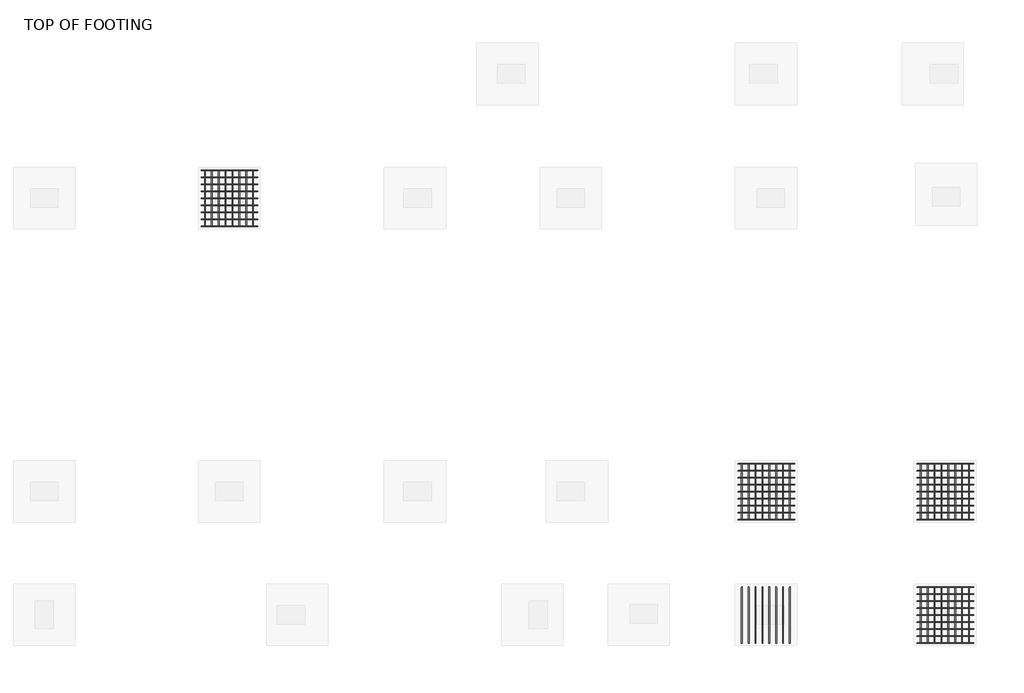
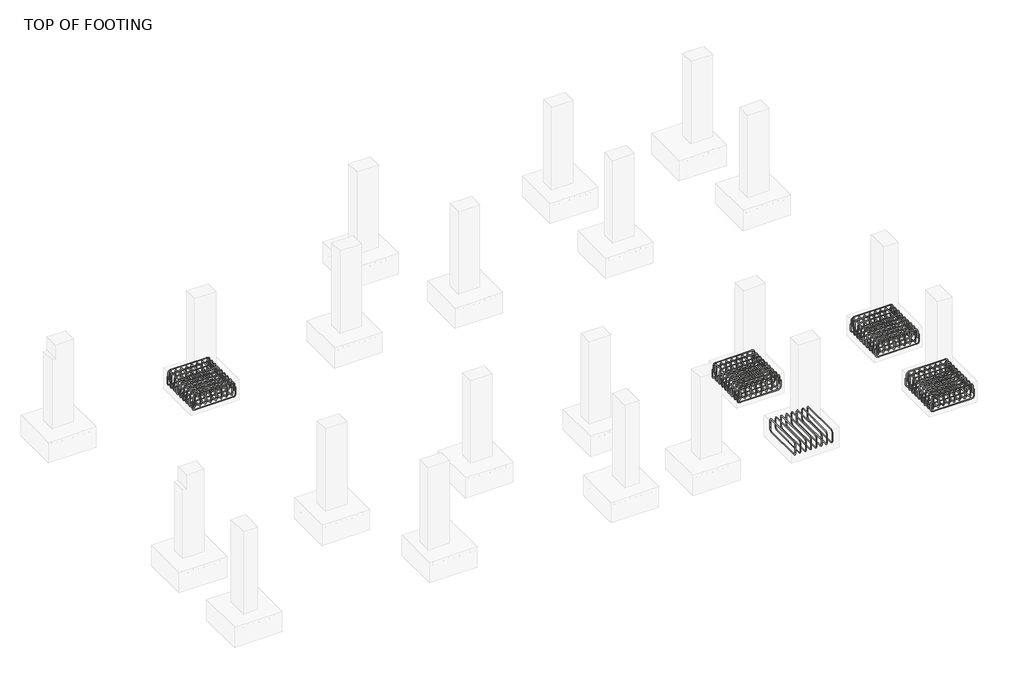
# One storey, part 8 of 20: 18 reinforcing bars.
"""IFC4 building model written with IfcOpenShell, lengths in millimetres."""

from ifc_helpers import new_model, si_unit, point, frame, origin, place, context, project, spatial, polyline, circle_curve, trimmed, segment, composite_curve, source, transform, mapped, element, save
from ifc_brep_helpers import swept_disk

model = new_model("IFC4")

# Units and contexts
model_context = context("Model", 3, world=origin())
ifc_project = project(units=[si_unit("LENGTHUNIT", "METRE", prefix="MILLI")], contexts=[model_context])

# Site, building, storey
site = spatial("IfcSite", under=ifc_project)
building = spatial("IfcBuilding", under=site)
storey = spatial("IfcBuildingStorey", under=building, Name="TOP OF FOOTING", Elevation=-1828.8)

# Reinforcing bars
placement = place(None, origin())
reinforcing_bar_shape = source(origin(), model_context, "Body", "SolidModel", [
    swept_disk(composite_curve([segment(polyline([(1628.3796816, -4547.9729916, -2006.6587682), (1628.3796816, -4547.9729916, -2153.9587682)]), True, "CONTINUOUS"), segment(trimmed(circle_curve(frame((1582.0296816, -4547.9729916, -2153.9587682), z_axis=(0.0, 1.0, 0.0), x_axis=(46.34999999999991, 0.0, 0.0)), 46.35), [point((1628.3796816, -4547.9729916, -2153.9587682))], [point((1582.0296816, -4547.9729916, -2200.3087682))], True, "CARTESIAN"), True, "CONTINUOUS"), segment(polyline([(1582.0296816, -4547.9729916, -2200.3087682), (767.4296816, -4547.9729916, -2200.3087682)]), True, "CONTINUOUS"), segment(trimmed(circle_curve(frame((767.4296816, -4547.9729916, -2153.9587682), z_axis=(0.0, 1.0, 0.0), x_axis=(0.0, 0.0, -46.34999999999991)), 46.35), [point((767.4296816, -4547.9729916, -2200.3087682))], [point((721.0796816, -4547.9729916, -2153.9587682))], True, "CARTESIAN"), True, "CONTINUOUS"), segment(polyline([(721.0796816, -4547.9729916, -2153.9587682), (721.0796816, -4547.9729916, -2006.6587682)]), True, "CONTINUOUS")], self_intersect=False), 6.35),
])
element("IfcReinforcingBar", 1, at=placement, inside=storey, context=model_context, shape_type="MappedRepresentation", body=[
    mapped(reinforcing_bar_shape, transform((0.0, 0.0, 0.0), x_axis=(1.0, 0.0, 0.0), y_axis=(0.0, 1.0, 0.0), z_axis=(0.0, 0.0, 1.0))),
    mapped(reinforcing_bar_shape, transform((0.0, -113.4125, 0.0), x_axis=(1.0, 0.0, 0.0), y_axis=(0.0, 1.0, 0.0), z_axis=(0.0, 0.0, 1.0))),
    mapped(reinforcing_bar_shape, transform((0.0, -226.825, 0.0), x_axis=(1.0, 0.0, 0.0), y_axis=(0.0, 1.0, 0.0), z_axis=(0.0, 0.0, 1.0))),
    mapped(reinforcing_bar_shape, transform((0.0, -340.2375, 0.0), x_axis=(1.0, 0.0, 0.0), y_axis=(0.0, 1.0, 0.0), z_axis=(0.0, 0.0, 1.0))),
    mapped(reinforcing_bar_shape, transform((0.0, -453.65, 0.0), x_axis=(1.0, 0.0, 0.0), y_axis=(0.0, 1.0, 0.0), z_axis=(0.0, 0.0, 1.0))),
    mapped(reinforcing_bar_shape, transform((0.0, -567.0625, 0.0), x_axis=(1.0, 0.0, 0.0), y_axis=(0.0, 1.0, 0.0), z_axis=(0.0, 0.0, 1.0))),
    mapped(reinforcing_bar_shape, transform((0.0, -680.475, 0.0), x_axis=(1.0, 0.0, 0.0), y_axis=(0.0, 1.0, 0.0), z_axis=(0.0, 0.0, 1.0))),
    mapped(reinforcing_bar_shape, transform((0.0, -793.8875, 0.0), x_axis=(1.0, 0.0, 0.0), y_axis=(0.0, 1.0, 0.0), z_axis=(0.0, 0.0, 1.0))),
    mapped(reinforcing_bar_shape, transform((0.0, -907.3, 0.0), x_axis=(1.0, 0.0, 0.0), y_axis=(0.0, 1.0, 0.0), z_axis=(0.0, 0.0, 1.0))),
])
reinforcing_bar_2_shape = source(origin(), model_context, "Body", "SolidModel", [
    swept_disk(composite_curve([segment(polyline([(740.553793, -4547.9729916, -2068.8), (740.553793, -4547.9729916, -1921.5)]), True, "CONTINUOUS"), segment(trimmed(circle_curve(frame((786.903793, -4547.9729916, -1921.5), z_axis=(0.0, 1.0, 0.0), x_axis=(-46.34999999999991, 0.0, 0.0)), 46.35), [point((740.553793, -4547.9729916, -1921.5))], [point((786.903793, -4547.9729916, -1875.15))], True, "CARTESIAN"), True, "CONTINUOUS"), segment(polyline([(786.903793, -4547.9729916, -1875.15), (1556.3671926, -4547.9729916, -1875.15)]), True, "CONTINUOUS"), segment(trimmed(circle_curve(frame((1556.3671926, -4547.9729916, -1921.5), z_axis=(0.0, 1.0, 0.0), x_axis=(0.0, 0.0, 46.34999999999991)), 46.35), [point((1556.3671926, -4547.9729916, -1875.15))], [point((1602.7171926, -4547.9729916, -1921.5))], True, "CARTESIAN"), True, "CONTINUOUS"), segment(polyline([(1602.7171926, -4547.9729916, -1921.5), (1602.7171926, -4547.9729916, -2068.8)]), True, "CONTINUOUS")], self_intersect=False), 6.35),
])
element("IfcReinforcingBar", 2, at=placement, inside=storey, context=model_context, shape_type="MappedRepresentation", body=[
    mapped(reinforcing_bar_2_shape, transform((0.0, 0.0, 0.0), x_axis=(1.0, 0.0, 0.0), y_axis=(0.0, 1.0, 0.0), z_axis=(0.0, 0.0, 1.0))),
    mapped(reinforcing_bar_2_shape, transform((0.0, -113.4125, 0.0), x_axis=(1.0, 0.0, 0.0), y_axis=(0.0, 1.0, 0.0), z_axis=(0.0, 0.0, 1.0))),
    mapped(reinforcing_bar_2_shape, transform((0.0, -226.825, 0.0), x_axis=(1.0, 0.0, 0.0), y_axis=(0.0, 1.0, 0.0), z_axis=(0.0, 0.0, 1.0))),
    mapped(reinforcing_bar_2_shape, transform((0.0, -340.2375, 0.0), x_axis=(1.0, 0.0, 0.0), y_axis=(0.0, 1.0, 0.0), z_axis=(0.0, 0.0, 1.0))),
    mapped(reinforcing_bar_2_shape, transform((0.0, -453.65, 0.0), x_axis=(1.0, 0.0, 0.0), y_axis=(0.0, 1.0, 0.0), z_axis=(0.0, 0.0, 1.0))),
    mapped(reinforcing_bar_2_shape, transform((0.0, -567.0625, 0.0), x_axis=(1.0, 0.0, 0.0), y_axis=(0.0, 1.0, 0.0), z_axis=(0.0, 0.0, 1.0))),
    mapped(reinforcing_bar_2_shape, transform((0.0, -680.475, 0.0), x_axis=(1.0, 0.0, 0.0), y_axis=(0.0, 1.0, 0.0), z_axis=(0.0, 0.0, 1.0))),
    mapped(reinforcing_bar_2_shape, transform((0.0, -793.8875, 0.0), x_axis=(1.0, 0.0, 0.0), y_axis=(0.0, 1.0, 0.0), z_axis=(0.0, 0.0, 1.0))),
    mapped(reinforcing_bar_2_shape, transform((0.0, -907.3, 0.0), x_axis=(1.0, 0.0, 0.0), y_axis=(0.0, 1.0, 0.0), z_axis=(0.0, 0.0, 1.0))),
])
reinforcing_bar_3_shape = source(origin(), model_context, "Body", "SolidModel", [
    swept_disk(composite_curve([segment(polyline([(1556.8827202, -4547.9729916, -2086.1951968), (1556.8827202, -4547.9729916, -1938.8951968)]), True, "CONTINUOUS"), segment(trimmed(circle_curve(frame((1556.8827202, -4594.3229916, -1938.8951968), z_axis=(1.0, 0.0, 0.0), x_axis=(0.0, 46.350000000000364, 0.0)), 46.35), [point((1556.8827202, -4547.9729916, -1938.8951968))], [point((1556.8827202, -4594.3229916, -1892.5451968))], True, "CARTESIAN"), True, "CONTINUOUS"), segment(polyline([(1556.8827202, -4594.3229916, -1892.5451968), (1556.8827202, -5408.9229916, -1892.5451968)]), True, "CONTINUOUS"), segment(trimmed(circle_curve(frame((1556.8827202, -5408.9229916, -1938.8951968), z_axis=(1.0, 0.0, 0.0), x_axis=(0.0, 0.0, 46.34999999999991)), 46.35), [point((1556.8827202, -5408.9229916, -1892.5451968))], [point((1556.8827202, -5455.2729916, -1938.8951968))], True, "CARTESIAN"), True, "CONTINUOUS"), segment(polyline([(1556.8827202, -5455.2729916, -1938.8951968), (1556.8827202, -5455.2729916, -2086.1951968)]), True, "CONTINUOUS")], self_intersect=False), 6.35),
])
element("IfcReinforcingBar", 3, at=placement, inside=storey, context=model_context, shape_type="MappedRepresentation", body=[
    mapped(reinforcing_bar_3_shape, transform((0.0, 0.0, 0.0), x_axis=(1.0, 0.0, 0.0), y_axis=(0.0, 1.0, 0.0), z_axis=(0.0, 0.0, 1.0))),
    mapped(reinforcing_bar_3_shape, transform((-111.2862402, 0.0, 0.0), x_axis=(1.0, 0.0, 0.0), y_axis=(0.0, 1.0, 0.0), z_axis=(0.0, 0.0, 1.0))),
    mapped(reinforcing_bar_3_shape, transform((-222.5724804, 0.0, 0.0), x_axis=(1.0, 0.0, 0.0), y_axis=(0.0, 1.0, 0.0), z_axis=(0.0, 0.0, 1.0))),
    mapped(reinforcing_bar_3_shape, transform((-333.8587205, 0.0, 0.0), x_axis=(1.0, 0.0, 0.0), y_axis=(0.0, 1.0, 0.0), z_axis=(0.0, 0.0, 1.0))),
    mapped(reinforcing_bar_3_shape, transform((-445.1449607, 0.0, 0.0), x_axis=(1.0, 0.0, 0.0), y_axis=(0.0, 1.0, 0.0), z_axis=(0.0, 0.0, 1.0))),
    mapped(reinforcing_bar_3_shape, transform((-556.4312009, 0.0, 0.0), x_axis=(1.0, 0.0, 0.0), y_axis=(0.0, 1.0, 0.0), z_axis=(0.0, 0.0, 1.0))),
    mapped(reinforcing_bar_3_shape, transform((-667.7174411, 0.0, 0.0), x_axis=(1.0, 0.0, 0.0), y_axis=(0.0, 1.0, 0.0), z_axis=(0.0, 0.0, 1.0))),
    mapped(reinforcing_bar_3_shape, transform((-779.0036813, 0.0, 0.0), x_axis=(1.0, 0.0, 0.0), y_axis=(0.0, 1.0, 0.0), z_axis=(0.0, 0.0, 1.0))),
])
reinforcing_bar_4_shape = source(origin(), model_context, "Body", "SolidModel", [
    swept_disk(composite_curve([segment(polyline([(777.879039, -4547.9729916, -1979.1645013), (777.879039, -4547.9729916, -2126.4645013)]), True, "CONTINUOUS"), segment(trimmed(circle_curve(frame((777.879039, -4594.3229916, -2126.4645013), z_axis=(-1.0, 0.0, 0.0), x_axis=(0.0, 46.350000000000364, 0.0)), 46.35), [point((777.879039, -4547.9729916, -2126.4645013))], [point((777.879039, -4594.3229916, -2172.8145013))], True, "CARTESIAN"), True, "CONTINUOUS"), segment(polyline([(777.879039, -4594.3229916, -2172.8145013), (777.879039, -5408.9229916, -2172.8145013)]), True, "CONTINUOUS"), segment(trimmed(circle_curve(frame((777.879039, -5408.9229916, -2126.4645013), z_axis=(-1.0, 0.0, 0.0), x_axis=(0.0, 0.0, -46.34999999999991)), 46.35), [point((777.879039, -5408.9229916, -2172.8145013))], [point((777.879039, -5455.2729916, -2126.4645013))], True, "CARTESIAN"), True, "CONTINUOUS"), segment(polyline([(777.879039, -5455.2729916, -2126.4645013), (777.879039, -5455.2729916, -1979.1645013)]), True, "CONTINUOUS")], self_intersect=False), 6.35),
])
element("IfcReinforcingBar", 4, at=placement, inside=storey, context=model_context, shape_type="MappedRepresentation", body=[
    mapped(reinforcing_bar_4_shape, transform((0.0, 0.0, 0.0), x_axis=(1.0, 0.0, 0.0), y_axis=(0.0, 1.0, 0.0), z_axis=(0.0, 0.0, 1.0))),
    mapped(reinforcing_bar_4_shape, transform((111.2862402, 0.0, 0.0), x_axis=(1.0, 0.0, 0.0), y_axis=(0.0, 1.0, 0.0), z_axis=(0.0, 0.0, 1.0))),
    mapped(reinforcing_bar_4_shape, transform((222.5724804, 0.0, 0.0), x_axis=(1.0, 0.0, 0.0), y_axis=(0.0, 1.0, 0.0), z_axis=(0.0, 0.0, 1.0))),
    mapped(reinforcing_bar_4_shape, transform((333.8587205, 0.0, 0.0), x_axis=(1.0, 0.0, 0.0), y_axis=(0.0, 1.0, 0.0), z_axis=(0.0, 0.0, 1.0))),
    mapped(reinforcing_bar_4_shape, transform((445.1449607, 0.0, 0.0), x_axis=(1.0, 0.0, 0.0), y_axis=(0.0, 1.0, 0.0), z_axis=(0.0, 0.0, 1.0))),
    mapped(reinforcing_bar_4_shape, transform((556.4312009, 0.0, 0.0), x_axis=(1.0, 0.0, 0.0), y_axis=(0.0, 1.0, 0.0), z_axis=(0.0, 0.0, 1.0))),
    mapped(reinforcing_bar_4_shape, transform((667.7174411, 0.0, 0.0), x_axis=(1.0, 0.0, 0.0), y_axis=(0.0, 1.0, 0.0), z_axis=(0.0, 0.0, 1.0))),
    mapped(reinforcing_bar_4_shape, transform((779.0036813, 0.0, 0.0), x_axis=(1.0, 0.0, 0.0), y_axis=(0.0, 1.0, 0.0), z_axis=(0.0, 0.0, 1.0))),
])
reinforcing_bar_5_shape = source(origin(), model_context, "Body", "SolidModel", [
    swept_disk(composite_curve([segment(polyline([(13222.7663908, -11304.2470059, -2006.6587682), (13222.7663908, -11304.2470059, -2153.9587682)]), True, "CONTINUOUS"), segment(trimmed(circle_curve(frame((13176.4163908, -11304.2470059, -2153.9587682), z_axis=(0.0, 1.0, 0.0), x_axis=(46.350000000000364, 0.0, 0.0)), 46.35), [point((13222.7663908, -11304.2470059, -2153.9587682))], [point((13176.4163908, -11304.2470059, -2200.3087682))], True, "CARTESIAN"), True, "CONTINUOUS"), segment(polyline([(13176.4163908, -11304.2470059, -2200.3087682), (12361.8163908, -11304.2470059, -2200.3087682)]), True, "CONTINUOUS"), segment(trimmed(circle_curve(frame((12361.8163908, -11304.2470059, -2153.9587682), z_axis=(0.0, 1.0, 0.0), x_axis=(0.0, 0.0, -46.34999999999991)), 46.35), [point((12361.8163908, -11304.2470059, -2200.3087682))], [point((12315.4663908, -11304.2470059, -2153.9587682))], True, "CARTESIAN"), True, "CONTINUOUS"), segment(polyline([(12315.4663908, -11304.2470059, -2153.9587682), (12315.4663908, -11304.2470059, -2006.6587682)]), True, "CONTINUOUS")], self_intersect=False), 6.35),
])
element("IfcReinforcingBar", 5, at=placement, inside=storey, context=model_context, shape_type="MappedRepresentation", body=[
    mapped(reinforcing_bar_5_shape, transform((0.0, 0.0, 0.0), x_axis=(1.0, 0.0, 0.0), y_axis=(0.0, 1.0, 0.0), z_axis=(0.0, 0.0, 1.0))),
    mapped(reinforcing_bar_5_shape, transform((0.0, -113.4125, 0.0), x_axis=(1.0, 0.0, 0.0), y_axis=(0.0, 1.0, 0.0), z_axis=(0.0, 0.0, 1.0))),
    mapped(reinforcing_bar_5_shape, transform((0.0, -226.825, 0.0), x_axis=(1.0, 0.0, 0.0), y_axis=(0.0, 1.0, 0.0), z_axis=(0.0, 0.0, 1.0))),
    mapped(reinforcing_bar_5_shape, transform((0.0, -340.2375, 0.0), x_axis=(1.0, 0.0, 0.0), y_axis=(0.0, 1.0, 0.0), z_axis=(0.0, 0.0, 1.0))),
    mapped(reinforcing_bar_5_shape, transform((0.0, -453.65, 0.0), x_axis=(1.0, 0.0, 0.0), y_axis=(0.0, 1.0, 0.0), z_axis=(0.0, 0.0, 1.0))),
    mapped(reinforcing_bar_5_shape, transform((0.0, -567.0625, 0.0), x_axis=(1.0, 0.0, 0.0), y_axis=(0.0, 1.0, 0.0), z_axis=(0.0, 0.0, 1.0))),
    mapped(reinforcing_bar_5_shape, transform((0.0, -680.475, 0.0), x_axis=(1.0, 0.0, 0.0), y_axis=(0.0, 1.0, 0.0), z_axis=(0.0, 0.0, 1.0))),
    mapped(reinforcing_bar_5_shape, transform((0.0, -793.8875, 0.0), x_axis=(1.0, 0.0, 0.0), y_axis=(0.0, 1.0, 0.0), z_axis=(0.0, 0.0, 1.0))),
    mapped(reinforcing_bar_5_shape, transform((0.0, -907.3, 0.0), x_axis=(1.0, 0.0, 0.0), y_axis=(0.0, 1.0, 0.0), z_axis=(0.0, 0.0, 1.0))),
])
reinforcing_bar_6_shape = source(origin(), model_context, "Body", "SolidModel", [
    swept_disk(composite_curve([segment(polyline([(12334.9405021, -11304.2470059, -2068.8), (12334.9405021, -11304.2470059, -1921.5)]), True, "CONTINUOUS"), segment(trimmed(circle_curve(frame((12381.2905021, -11304.2470059, -1921.5), z_axis=(0.0, 1.0, 0.0), x_axis=(-46.350000000000364, 0.0, 0.0)), 46.35), [point((12334.9405021, -11304.2470059, -1921.5))], [point((12381.2905021, -11304.2470059, -1875.15))], True, "CARTESIAN"), True, "CONTINUOUS"), segment(polyline([(12381.2905021, -11304.2470059, -1875.15), (13150.7539017, -11304.2470059, -1875.15)]), True, "CONTINUOUS"), segment(trimmed(circle_curve(frame((13150.7539017, -11304.2470059, -1921.5), z_axis=(0.0, 1.0, 0.0), x_axis=(0.0, 0.0, 46.34999999999991)), 46.35), [point((13150.7539017, -11304.2470059, -1875.15))], [point((13197.1039017, -11304.2470059, -1921.5))], True, "CARTESIAN"), True, "CONTINUOUS"), segment(polyline([(13197.1039017, -11304.2470059, -1921.5), (13197.1039017, -11304.2470059, -2068.8)]), True, "CONTINUOUS")], self_intersect=False), 6.35),
])
element("IfcReinforcingBar", 6, at=placement, inside=storey, context=model_context, shape_type="MappedRepresentation", body=[
    mapped(reinforcing_bar_6_shape, transform((0.0, 0.0, 0.0), x_axis=(1.0, 0.0, 0.0), y_axis=(0.0, 1.0, 0.0), z_axis=(0.0, 0.0, 1.0))),
    mapped(reinforcing_bar_6_shape, transform((0.0, -113.4125, 0.0), x_axis=(1.0, 0.0, 0.0), y_axis=(0.0, 1.0, 0.0), z_axis=(0.0, 0.0, 1.0))),
    mapped(reinforcing_bar_6_shape, transform((0.0, -226.825, 0.0), x_axis=(1.0, 0.0, 0.0), y_axis=(0.0, 1.0, 0.0), z_axis=(0.0, 0.0, 1.0))),
    mapped(reinforcing_bar_6_shape, transform((0.0, -340.2375, 0.0), x_axis=(1.0, 0.0, 0.0), y_axis=(0.0, 1.0, 0.0), z_axis=(0.0, 0.0, 1.0))),
    mapped(reinforcing_bar_6_shape, transform((0.0, -453.65, 0.0), x_axis=(1.0, 0.0, 0.0), y_axis=(0.0, 1.0, 0.0), z_axis=(0.0, 0.0, 1.0))),
    mapped(reinforcing_bar_6_shape, transform((0.0, -567.0625, 0.0), x_axis=(1.0, 0.0, 0.0), y_axis=(0.0, 1.0, 0.0), z_axis=(0.0, 0.0, 1.0))),
    mapped(reinforcing_bar_6_shape, transform((0.0, -680.475, 0.0), x_axis=(1.0, 0.0, 0.0), y_axis=(0.0, 1.0, 0.0), z_axis=(0.0, 0.0, 1.0))),
    mapped(reinforcing_bar_6_shape, transform((0.0, -793.8875, 0.0), x_axis=(1.0, 0.0, 0.0), y_axis=(0.0, 1.0, 0.0), z_axis=(0.0, 0.0, 1.0))),
    mapped(reinforcing_bar_6_shape, transform((0.0, -907.3, 0.0), x_axis=(1.0, 0.0, 0.0), y_axis=(0.0, 1.0, 0.0), z_axis=(0.0, 0.0, 1.0))),
])
reinforcing_bar_7_shape = source(origin(), model_context, "Body", "SolidModel", [
    swept_disk(composite_curve([segment(polyline([(13151.2694294, -11304.2470059, -2086.1951968), (13151.2694294, -11304.2470059, -1938.8951968)]), True, "CONTINUOUS"), segment(trimmed(circle_curve(frame((13151.2694294, -11350.5970059, -1938.8951968), z_axis=(1.0, 0.0, 0.0), x_axis=(0.0, 46.349999999998545, 0.0)), 46.35), [point((13151.2694294, -11304.2470059, -1938.8951968))], [point((13151.2694294, -11350.5970059, -1892.5451968))], True, "CARTESIAN"), True, "CONTINUOUS"), segment(polyline([(13151.2694294, -11350.5970059, -1892.5451968), (13151.2694294, -12165.1970059, -1892.5451968)]), True, "CONTINUOUS"), segment(trimmed(circle_curve(frame((13151.2694294, -12165.1970059, -1938.8951968), z_axis=(1.0, 0.0, 0.0), x_axis=(0.0, 0.0, 46.34999999999991)), 46.35), [point((13151.2694294, -12165.1970059, -1892.5451968))], [point((13151.2694294, -12211.5470059, -1938.8951968))], True, "CARTESIAN"), True, "CONTINUOUS"), segment(polyline([(13151.2694294, -12211.5470059, -1938.8951968), (13151.2694294, -12211.5470059, -2086.1951968)]), True, "CONTINUOUS")], self_intersect=False), 6.35),
])
element("IfcReinforcingBar", 7, at=placement, inside=storey, context=model_context, shape_type="MappedRepresentation", body=[
    mapped(reinforcing_bar_7_shape, transform((0.0, 0.0, 0.0), x_axis=(1.0, 0.0, 0.0), y_axis=(0.0, 1.0, 0.0), z_axis=(0.0, 0.0, 1.0))),
    mapped(reinforcing_bar_7_shape, transform((-111.2862402, 0.0, 0.0), x_axis=(1.0, 0.0, 0.0), y_axis=(0.0, 1.0, 0.0), z_axis=(0.0, 0.0, 1.0))),
    mapped(reinforcing_bar_7_shape, transform((-222.5724804, 0.0, 0.0), x_axis=(1.0, 0.0, 0.0), y_axis=(0.0, 1.0, 0.0), z_axis=(0.0, 0.0, 1.0))),
    mapped(reinforcing_bar_7_shape, transform((-333.8587205, 0.0, 0.0), x_axis=(1.0, 0.0, 0.0), y_axis=(0.0, 1.0, 0.0), z_axis=(0.0, 0.0, 1.0))),
    mapped(reinforcing_bar_7_shape, transform((-445.1449607, 0.0, 0.0), x_axis=(1.0, 0.0, 0.0), y_axis=(0.0, 1.0, 0.0), z_axis=(0.0, 0.0, 1.0))),
    mapped(reinforcing_bar_7_shape, transform((-556.4312009, 0.0, 0.0), x_axis=(1.0, 0.0, 0.0), y_axis=(0.0, 1.0, 0.0), z_axis=(0.0, 0.0, 1.0))),
    mapped(reinforcing_bar_7_shape, transform((-667.7174411, 0.0, 0.0), x_axis=(1.0, 0.0, 0.0), y_axis=(0.0, 1.0, 0.0), z_axis=(0.0, 0.0, 1.0))),
    mapped(reinforcing_bar_7_shape, transform((-779.0036813, 0.0, 0.0), x_axis=(1.0, 0.0, 0.0), y_axis=(0.0, 1.0, 0.0), z_axis=(0.0, 0.0, 1.0))),
])
reinforcing_bar_8_shape = source(origin(), model_context, "Body", "SolidModel", [
    swept_disk(composite_curve([segment(polyline([(12372.2657481, -11304.2470059, -1979.1645013), (12372.2657481, -11304.2470059, -2126.4645013)]), True, "CONTINUOUS"), segment(trimmed(circle_curve(frame((12372.2657481, -11350.5970059, -2126.4645013), z_axis=(-1.0, 0.0, 0.0), x_axis=(0.0, 46.349999999998545, 0.0)), 46.35), [point((12372.2657481, -11304.2470059, -2126.4645013))], [point((12372.2657481, -11350.5970059, -2172.8145013))], True, "CARTESIAN"), True, "CONTINUOUS"), segment(polyline([(12372.2657481, -11350.5970059, -2172.8145013), (12372.2657481, -12165.1970059, -2172.8145013)]), True, "CONTINUOUS"), segment(trimmed(circle_curve(frame((12372.2657481, -12165.1970059, -2126.4645013), z_axis=(-1.0, 0.0, 0.0), x_axis=(0.0, 0.0, -46.34999999999991)), 46.35), [point((12372.2657481, -12165.1970059, -2172.8145013))], [point((12372.2657481, -12211.5470059, -2126.4645013))], True, "CARTESIAN"), True, "CONTINUOUS"), segment(polyline([(12372.2657481, -12211.5470059, -2126.4645013), (12372.2657481, -12211.5470059, -1979.1645013)]), True, "CONTINUOUS")], self_intersect=False), 6.35),
])
element("IfcReinforcingBar", 8, at=placement, inside=storey, context=model_context, shape_type="MappedRepresentation", body=[
    mapped(reinforcing_bar_8_shape, transform((0.0, 0.0, 0.0), x_axis=(1.0, 0.0, 0.0), y_axis=(0.0, 1.0, 0.0), z_axis=(0.0, 0.0, 1.0))),
    mapped(reinforcing_bar_8_shape, transform((111.2862402, 0.0, 0.0), x_axis=(1.0, 0.0, 0.0), y_axis=(0.0, 1.0, 0.0), z_axis=(0.0, 0.0, 1.0))),
    mapped(reinforcing_bar_8_shape, transform((222.5724804, 0.0, 0.0), x_axis=(1.0, 0.0, 0.0), y_axis=(0.0, 1.0, 0.0), z_axis=(0.0, 0.0, 1.0))),
    mapped(reinforcing_bar_8_shape, transform((333.8587205, 0.0, 0.0), x_axis=(1.0, 0.0, 0.0), y_axis=(0.0, 1.0, 0.0), z_axis=(0.0, 0.0, 1.0))),
    mapped(reinforcing_bar_8_shape, transform((445.1449607, 0.0, 0.0), x_axis=(1.0, 0.0, 0.0), y_axis=(0.0, 1.0, 0.0), z_axis=(0.0, 0.0, 1.0))),
    mapped(reinforcing_bar_8_shape, transform((556.4312009, 0.0, 0.0), x_axis=(1.0, 0.0, 0.0), y_axis=(0.0, 1.0, 0.0), z_axis=(0.0, 0.0, 1.0))),
    mapped(reinforcing_bar_8_shape, transform((667.7174411, 0.0, 0.0), x_axis=(1.0, 0.0, 0.0), y_axis=(0.0, 1.0, 0.0), z_axis=(0.0, 0.0, 1.0))),
    mapped(reinforcing_bar_8_shape, transform((779.0036813, 0.0, 0.0), x_axis=(1.0, 0.0, 0.0), y_axis=(0.0, 1.0, 0.0), z_axis=(0.0, 0.0, 1.0))),
])
reinforcing_bar_9_shape = source(origin(), model_context, "Body", "SolidModel", [
    swept_disk(composite_curve([segment(polyline([(13222.7663908, -9303.4578267, -2006.6587682), (13222.7663908, -9303.4578267, -2153.9587682)]), True, "CONTINUOUS"), segment(trimmed(circle_curve(frame((13176.4163908, -9303.4578267, -2153.9587682), z_axis=(0.0, 1.0, 0.0), x_axis=(46.350000000000364, 0.0, 0.0)), 46.35), [point((13222.7663908, -9303.4578267, -2153.9587682))], [point((13176.4163908, -9303.4578267, -2200.3087682))], True, "CARTESIAN"), True, "CONTINUOUS"), segment(polyline([(13176.4163908, -9303.4578267, -2200.3087682), (12361.8163908, -9303.4578267, -2200.3087682)]), True, "CONTINUOUS"), segment(trimmed(circle_curve(frame((12361.8163908, -9303.4578267, -2153.9587682), z_axis=(0.0, 1.0, 0.0), x_axis=(0.0, 0.0, -46.34999999999991)), 46.35), [point((12361.8163908, -9303.4578267, -2200.3087682))], [point((12315.4663908, -9303.4578267, -2153.9587682))], True, "CARTESIAN"), True, "CONTINUOUS"), segment(polyline([(12315.4663908, -9303.4578267, -2153.9587682), (12315.4663908, -9303.4578267, -2006.6587682)]), True, "CONTINUOUS")], self_intersect=False), 6.35),
])
element("IfcReinforcingBar", 9, at=placement, inside=storey, context=model_context, shape_type="MappedRepresentation", body=[
    mapped(reinforcing_bar_9_shape, transform((0.0, 0.0, 0.0), x_axis=(1.0, 0.0, 0.0), y_axis=(0.0, 1.0, 0.0), z_axis=(0.0, 0.0, 1.0))),
    mapped(reinforcing_bar_9_shape, transform((0.0, -113.4125, 0.0), x_axis=(1.0, 0.0, 0.0), y_axis=(0.0, 1.0, 0.0), z_axis=(0.0, 0.0, 1.0))),
    mapped(reinforcing_bar_9_shape, transform((0.0, -226.825, 0.0), x_axis=(1.0, 0.0, 0.0), y_axis=(0.0, 1.0, 0.0), z_axis=(0.0, 0.0, 1.0))),
    mapped(reinforcing_bar_9_shape, transform((0.0, -340.2375, 0.0), x_axis=(1.0, 0.0, 0.0), y_axis=(0.0, 1.0, 0.0), z_axis=(0.0, 0.0, 1.0))),
    mapped(reinforcing_bar_9_shape, transform((0.0, -453.65, 0.0), x_axis=(1.0, 0.0, 0.0), y_axis=(0.0, 1.0, 0.0), z_axis=(0.0, 0.0, 1.0))),
    mapped(reinforcing_bar_9_shape, transform((0.0, -567.0625, 0.0), x_axis=(1.0, 0.0, 0.0), y_axis=(0.0, 1.0, 0.0), z_axis=(0.0, 0.0, 1.0))),
    mapped(reinforcing_bar_9_shape, transform((0.0, -680.475, 0.0), x_axis=(1.0, 0.0, 0.0), y_axis=(0.0, 1.0, 0.0), z_axis=(0.0, 0.0, 1.0))),
    mapped(reinforcing_bar_9_shape, transform((0.0, -793.8875, 0.0), x_axis=(1.0, 0.0, 0.0), y_axis=(0.0, 1.0, 0.0), z_axis=(0.0, 0.0, 1.0))),
    mapped(reinforcing_bar_9_shape, transform((0.0, -907.3, 0.0), x_axis=(1.0, 0.0, 0.0), y_axis=(0.0, 1.0, 0.0), z_axis=(0.0, 0.0, 1.0))),
])
reinforcing_bar_10_shape = source(origin(), model_context, "Body", "SolidModel", [
    swept_disk(composite_curve([segment(polyline([(12334.9405021, -9303.4578267, -2068.8), (12334.9405021, -9303.4578267, -1921.5)]), True, "CONTINUOUS"), segment(trimmed(circle_curve(frame((12381.2905021, -9303.4578267, -1921.5), z_axis=(0.0, 1.0, 0.0), x_axis=(-46.350000000000364, 0.0, 0.0)), 46.35), [point((12334.9405021, -9303.4578267, -1921.5))], [point((12381.2905021, -9303.4578267, -1875.15))], True, "CARTESIAN"), True, "CONTINUOUS"), segment(polyline([(12381.2905021, -9303.4578267, -1875.15), (13150.7539017, -9303.4578267, -1875.15)]), True, "CONTINUOUS"), segment(trimmed(circle_curve(frame((13150.7539017, -9303.4578267, -1921.5), z_axis=(0.0, 1.0, 0.0), x_axis=(0.0, 0.0, 46.34999999999991)), 46.35), [point((13150.7539017, -9303.4578267, -1875.15))], [point((13197.1039017, -9303.4578267, -1921.5))], True, "CARTESIAN"), True, "CONTINUOUS"), segment(polyline([(13197.1039017, -9303.4578267, -1921.5), (13197.1039017, -9303.4578267, -2068.8)]), True, "CONTINUOUS")], self_intersect=False), 6.35),
])
element("IfcReinforcingBar", 10, at=placement, inside=storey, context=model_context, shape_type="MappedRepresentation", body=[
    mapped(reinforcing_bar_10_shape, transform((0.0, 0.0, 0.0), x_axis=(1.0, 0.0, 0.0), y_axis=(0.0, 1.0, 0.0), z_axis=(0.0, 0.0, 1.0))),
    mapped(reinforcing_bar_10_shape, transform((0.0, -113.4125, 0.0), x_axis=(1.0, 0.0, 0.0), y_axis=(0.0, 1.0, 0.0), z_axis=(0.0, 0.0, 1.0))),
    mapped(reinforcing_bar_10_shape, transform((0.0, -226.825, 0.0), x_axis=(1.0, 0.0, 0.0), y_axis=(0.0, 1.0, 0.0), z_axis=(0.0, 0.0, 1.0))),
    mapped(reinforcing_bar_10_shape, transform((0.0, -340.2375, 0.0), x_axis=(1.0, 0.0, 0.0), y_axis=(0.0, 1.0, 0.0), z_axis=(0.0, 0.0, 1.0))),
    mapped(reinforcing_bar_10_shape, transform((0.0, -453.65, 0.0), x_axis=(1.0, 0.0, 0.0), y_axis=(0.0, 1.0, 0.0), z_axis=(0.0, 0.0, 1.0))),
    mapped(reinforcing_bar_10_shape, transform((0.0, -567.0625, 0.0), x_axis=(1.0, 0.0, 0.0), y_axis=(0.0, 1.0, 0.0), z_axis=(0.0, 0.0, 1.0))),
    mapped(reinforcing_bar_10_shape, transform((0.0, -680.475, 0.0), x_axis=(1.0, 0.0, 0.0), y_axis=(0.0, 1.0, 0.0), z_axis=(0.0, 0.0, 1.0))),
    mapped(reinforcing_bar_10_shape, transform((0.0, -793.8875, 0.0), x_axis=(1.0, 0.0, 0.0), y_axis=(0.0, 1.0, 0.0), z_axis=(0.0, 0.0, 1.0))),
    mapped(reinforcing_bar_10_shape, transform((0.0, -907.3, 0.0), x_axis=(1.0, 0.0, 0.0), y_axis=(0.0, 1.0, 0.0), z_axis=(0.0, 0.0, 1.0))),
])
reinforcing_bar_11_shape = source(origin(), model_context, "Body", "SolidModel", [
    swept_disk(composite_curve([segment(polyline([(13151.2694294, -9303.4578267, -2086.1951968), (13151.2694294, -9303.4578267, -1938.8951968)]), True, "CONTINUOUS"), segment(trimmed(circle_curve(frame((13151.2694294, -9349.8078267, -1938.8951968), z_axis=(1.0, 0.0, 0.0), x_axis=(0.0, 46.350000000000364, 0.0)), 46.35), [point((13151.2694294, -9303.4578267, -1938.8951968))], [point((13151.2694294, -9349.8078267, -1892.5451968))], True, "CARTESIAN"), True, "CONTINUOUS"), segment(polyline([(13151.2694294, -9349.8078267, -1892.5451968), (13151.2694294, -10164.4078267, -1892.5451968)]), True, "CONTINUOUS"), segment(trimmed(circle_curve(frame((13151.2694294, -10164.4078267, -1938.8951968), z_axis=(1.0, 0.0, 0.0), x_axis=(0.0, 0.0, 46.34999999999991)), 46.35), [point((13151.2694294, -10164.4078267, -1892.5451968))], [point((13151.2694294, -10210.7578267, -1938.8951968))], True, "CARTESIAN"), True, "CONTINUOUS"), segment(polyline([(13151.2694294, -10210.7578267, -1938.8951968), (13151.2694294, -10210.7578267, -2086.1951968)]), True, "CONTINUOUS")], self_intersect=False), 6.35),
])
element("IfcReinforcingBar", 11, at=placement, inside=storey, context=model_context, shape_type="MappedRepresentation", body=[
    mapped(reinforcing_bar_11_shape, transform((0.0, 0.0, 0.0), x_axis=(1.0, 0.0, 0.0), y_axis=(0.0, 1.0, 0.0), z_axis=(0.0, 0.0, 1.0))),
    mapped(reinforcing_bar_11_shape, transform((-111.2862402, 0.0, 0.0), x_axis=(1.0, 0.0, 0.0), y_axis=(0.0, 1.0, 0.0), z_axis=(0.0, 0.0, 1.0))),
    mapped(reinforcing_bar_11_shape, transform((-222.5724804, 0.0, 0.0), x_axis=(1.0, 0.0, 0.0), y_axis=(0.0, 1.0, 0.0), z_axis=(0.0, 0.0, 1.0))),
    mapped(reinforcing_bar_11_shape, transform((-333.8587205, 0.0, 0.0), x_axis=(1.0, 0.0, 0.0), y_axis=(0.0, 1.0, 0.0), z_axis=(0.0, 0.0, 1.0))),
    mapped(reinforcing_bar_11_shape, transform((-445.1449607, 0.0, 0.0), x_axis=(1.0, 0.0, 0.0), y_axis=(0.0, 1.0, 0.0), z_axis=(0.0, 0.0, 1.0))),
    mapped(reinforcing_bar_11_shape, transform((-556.4312009, 0.0, 0.0), x_axis=(1.0, 0.0, 0.0), y_axis=(0.0, 1.0, 0.0), z_axis=(0.0, 0.0, 1.0))),
    mapped(reinforcing_bar_11_shape, transform((-667.7174411, 0.0, 0.0), x_axis=(1.0, 0.0, 0.0), y_axis=(0.0, 1.0, 0.0), z_axis=(0.0, 0.0, 1.0))),
    mapped(reinforcing_bar_11_shape, transform((-779.0036813, 0.0, 0.0), x_axis=(1.0, 0.0, 0.0), y_axis=(0.0, 1.0, 0.0), z_axis=(0.0, 0.0, 1.0))),
])
reinforcing_bar_12_shape = source(origin(), model_context, "Body", "SolidModel", [
    swept_disk(composite_curve([segment(polyline([(12372.2657481, -9303.4578267, -1979.1645013), (12372.2657481, -9303.4578267, -2126.4645013)]), True, "CONTINUOUS"), segment(trimmed(circle_curve(frame((12372.2657481, -9349.8078267, -2126.4645013), z_axis=(-1.0, 0.0, 0.0), x_axis=(0.0, 46.350000000000364, 0.0)), 46.35), [point((12372.2657481, -9303.4578267, -2126.4645013))], [point((12372.2657481, -9349.8078267, -2172.8145013))], True, "CARTESIAN"), True, "CONTINUOUS"), segment(polyline([(12372.2657481, -9349.8078267, -2172.8145013), (12372.2657481, -10164.4078267, -2172.8145013)]), True, "CONTINUOUS"), segment(trimmed(circle_curve(frame((12372.2657481, -10164.4078267, -2126.4645013), z_axis=(-1.0, 0.0, 0.0), x_axis=(0.0, 0.0, -46.34999999999991)), 46.35), [point((12372.2657481, -10164.4078267, -2172.8145013))], [point((12372.2657481, -10210.7578267, -2126.4645013))], True, "CARTESIAN"), True, "CONTINUOUS"), segment(polyline([(12372.2657481, -10210.7578267, -2126.4645013), (12372.2657481, -10210.7578267, -1979.1645013)]), True, "CONTINUOUS")], self_intersect=False), 6.35),
])
element("IfcReinforcingBar", 12, at=placement, inside=storey, context=model_context, shape_type="MappedRepresentation", body=[
    mapped(reinforcing_bar_12_shape, transform((0.0, 0.0, 0.0), x_axis=(1.0, 0.0, 0.0), y_axis=(0.0, 1.0, 0.0), z_axis=(0.0, 0.0, 1.0))),
    mapped(reinforcing_bar_12_shape, transform((111.2862402, 0.0, 0.0), x_axis=(1.0, 0.0, 0.0), y_axis=(0.0, 1.0, 0.0), z_axis=(0.0, 0.0, 1.0))),
    mapped(reinforcing_bar_12_shape, transform((222.5724804, 0.0, 0.0), x_axis=(1.0, 0.0, 0.0), y_axis=(0.0, 1.0, 0.0), z_axis=(0.0, 0.0, 1.0))),
    mapped(reinforcing_bar_12_shape, transform((333.8587205, 0.0, 0.0), x_axis=(1.0, 0.0, 0.0), y_axis=(0.0, 1.0, 0.0), z_axis=(0.0, 0.0, 1.0))),
    mapped(reinforcing_bar_12_shape, transform((445.1449607, 0.0, 0.0), x_axis=(1.0, 0.0, 0.0), y_axis=(0.0, 1.0, 0.0), z_axis=(0.0, 0.0, 1.0))),
    mapped(reinforcing_bar_12_shape, transform((556.4312009, 0.0, 0.0), x_axis=(1.0, 0.0, 0.0), y_axis=(0.0, 1.0, 0.0), z_axis=(0.0, 0.0, 1.0))),
    mapped(reinforcing_bar_12_shape, transform((667.7174411, 0.0, 0.0), x_axis=(1.0, 0.0, 0.0), y_axis=(0.0, 1.0, 0.0), z_axis=(0.0, 0.0, 1.0))),
    mapped(reinforcing_bar_12_shape, transform((779.0036813, 0.0, 0.0), x_axis=(1.0, 0.0, 0.0), y_axis=(0.0, 1.0, 0.0), z_axis=(0.0, 0.0, 1.0))),
])
reinforcing_bar_13_shape = source(origin(), model_context, "Body", "SolidModel", [
    swept_disk(composite_curve([segment(polyline([(10322.7663908, -9303.4578267, -2006.6587682), (10322.7663908, -9303.4578267, -2153.9587682)]), True, "CONTINUOUS"), segment(trimmed(circle_curve(frame((10276.4163908, -9303.4578267, -2153.9587682), z_axis=(0.0, 1.0, 0.0), x_axis=(46.350000000000364, 0.0, 0.0)), 46.35), [point((10322.7663908, -9303.4578267, -2153.9587682))], [point((10276.4163908, -9303.4578267, -2200.3087682))], True, "CARTESIAN"), True, "CONTINUOUS"), segment(polyline([(10276.4163908, -9303.4578267, -2200.3087682), (9461.8163908, -9303.4578267, -2200.3087682)]), True, "CONTINUOUS"), segment(trimmed(circle_curve(frame((9461.8163908, -9303.4578267, -2153.9587682), z_axis=(0.0, 1.0, 0.0), x_axis=(0.0, 0.0, -46.34999999999991)), 46.35), [point((9461.8163908, -9303.4578267, -2200.3087682))], [point((9415.4663908, -9303.4578267, -2153.9587682))], True, "CARTESIAN"), True, "CONTINUOUS"), segment(polyline([(9415.4663908, -9303.4578267, -2153.9587682), (9415.4663908, -9303.4578267, -2006.6587682)]), True, "CONTINUOUS")], self_intersect=False), 6.35),
])
element("IfcReinforcingBar", 13, at=placement, inside=storey, context=model_context, shape_type="MappedRepresentation", body=[
    mapped(reinforcing_bar_13_shape, transform((0.0, 0.0, 0.0), x_axis=(1.0, 0.0, 0.0), y_axis=(0.0, 1.0, 0.0), z_axis=(0.0, 0.0, 1.0))),
    mapped(reinforcing_bar_13_shape, transform((0.0, -113.4125, 0.0), x_axis=(1.0, 0.0, 0.0), y_axis=(0.0, 1.0, 0.0), z_axis=(0.0, 0.0, 1.0))),
    mapped(reinforcing_bar_13_shape, transform((0.0, -226.825, 0.0), x_axis=(1.0, 0.0, 0.0), y_axis=(0.0, 1.0, 0.0), z_axis=(0.0, 0.0, 1.0))),
    mapped(reinforcing_bar_13_shape, transform((0.0, -340.2375, 0.0), x_axis=(1.0, 0.0, 0.0), y_axis=(0.0, 1.0, 0.0), z_axis=(0.0, 0.0, 1.0))),
    mapped(reinforcing_bar_13_shape, transform((0.0, -453.65, 0.0), x_axis=(1.0, 0.0, 0.0), y_axis=(0.0, 1.0, 0.0), z_axis=(0.0, 0.0, 1.0))),
    mapped(reinforcing_bar_13_shape, transform((0.0, -567.0625, 0.0), x_axis=(1.0, 0.0, 0.0), y_axis=(0.0, 1.0, 0.0), z_axis=(0.0, 0.0, 1.0))),
    mapped(reinforcing_bar_13_shape, transform((0.0, -680.475, 0.0), x_axis=(1.0, 0.0, 0.0), y_axis=(0.0, 1.0, 0.0), z_axis=(0.0, 0.0, 1.0))),
    mapped(reinforcing_bar_13_shape, transform((0.0, -793.8875, 0.0), x_axis=(1.0, 0.0, 0.0), y_axis=(0.0, 1.0, 0.0), z_axis=(0.0, 0.0, 1.0))),
    mapped(reinforcing_bar_13_shape, transform((0.0, -907.3, 0.0), x_axis=(1.0, 0.0, 0.0), y_axis=(0.0, 1.0, 0.0), z_axis=(0.0, 0.0, 1.0))),
])
reinforcing_bar_14_shape = source(origin(), model_context, "Body", "SolidModel", [
    swept_disk(composite_curve([segment(polyline([(9434.9405021, -9303.4578267, -2068.8), (9434.9405021, -9303.4578267, -1921.5)]), True, "CONTINUOUS"), segment(trimmed(circle_curve(frame((9481.2905021, -9303.4578267, -1921.5), z_axis=(0.0, 1.0, 0.0), x_axis=(-46.350000000000364, 0.0, 0.0)), 46.35), [point((9434.9405021, -9303.4578267, -1921.5))], [point((9481.2905021, -9303.4578267, -1875.15))], True, "CARTESIAN"), True, "CONTINUOUS"), segment(polyline([(9481.2905021, -9303.4578267, -1875.15), (10250.7539017, -9303.4578267, -1875.15)]), True, "CONTINUOUS"), segment(trimmed(circle_curve(frame((10250.7539017, -9303.4578267, -1921.5), z_axis=(0.0, 1.0, 0.0), x_axis=(0.0, 0.0, 46.34999999999991)), 46.35), [point((10250.7539017, -9303.4578267, -1875.15))], [point((10297.1039017, -9303.4578267, -1921.5))], True, "CARTESIAN"), True, "CONTINUOUS"), segment(polyline([(10297.1039017, -9303.4578267, -1921.5), (10297.1039017, -9303.4578267, -2068.8)]), True, "CONTINUOUS")], self_intersect=False), 6.35),
])
element("IfcReinforcingBar", 14, at=placement, inside=storey, context=model_context, shape_type="MappedRepresentation", body=[
    mapped(reinforcing_bar_14_shape, transform((0.0, 0.0, 0.0), x_axis=(1.0, 0.0, 0.0), y_axis=(0.0, 1.0, 0.0), z_axis=(0.0, 0.0, 1.0))),
    mapped(reinforcing_bar_14_shape, transform((0.0, -113.4125, 0.0), x_axis=(1.0, 0.0, 0.0), y_axis=(0.0, 1.0, 0.0), z_axis=(0.0, 0.0, 1.0))),
    mapped(reinforcing_bar_14_shape, transform((0.0, -226.825, 0.0), x_axis=(1.0, 0.0, 0.0), y_axis=(0.0, 1.0, 0.0), z_axis=(0.0, 0.0, 1.0))),
    mapped(reinforcing_bar_14_shape, transform((0.0, -340.2375, 0.0), x_axis=(1.0, 0.0, 0.0), y_axis=(0.0, 1.0, 0.0), z_axis=(0.0, 0.0, 1.0))),
    mapped(reinforcing_bar_14_shape, transform((0.0, -453.65, 0.0), x_axis=(1.0, 0.0, 0.0), y_axis=(0.0, 1.0, 0.0), z_axis=(0.0, 0.0, 1.0))),
    mapped(reinforcing_bar_14_shape, transform((0.0, -567.0625, 0.0), x_axis=(1.0, 0.0, 0.0), y_axis=(0.0, 1.0, 0.0), z_axis=(0.0, 0.0, 1.0))),
    mapped(reinforcing_bar_14_shape, transform((0.0, -680.475, 0.0), x_axis=(1.0, 0.0, 0.0), y_axis=(0.0, 1.0, 0.0), z_axis=(0.0, 0.0, 1.0))),
    mapped(reinforcing_bar_14_shape, transform((0.0, -793.8875, 0.0), x_axis=(1.0, 0.0, 0.0), y_axis=(0.0, 1.0, 0.0), z_axis=(0.0, 0.0, 1.0))),
    mapped(reinforcing_bar_14_shape, transform((0.0, -907.3, 0.0), x_axis=(1.0, 0.0, 0.0), y_axis=(0.0, 1.0, 0.0), z_axis=(0.0, 0.0, 1.0))),
])
reinforcing_bar_15_shape = source(origin(), model_context, "Body", "SolidModel", [
    swept_disk(composite_curve([segment(polyline([(10251.2694294, -9303.4578267, -2086.1951968), (10251.2694294, -9303.4578267, -1938.8951968)]), True, "CONTINUOUS"), segment(trimmed(circle_curve(frame((10251.2694294, -9349.8078267, -1938.8951968), z_axis=(1.0, 0.0, 0.0), x_axis=(0.0, 46.350000000000364, 0.0)), 46.35), [point((10251.2694294, -9303.4578267, -1938.8951968))], [point((10251.2694294, -9349.8078267, -1892.5451968))], True, "CARTESIAN"), True, "CONTINUOUS"), segment(polyline([(10251.2694294, -9349.8078267, -1892.5451968), (10251.2694294, -10164.4078267, -1892.5451968)]), True, "CONTINUOUS"), segment(trimmed(circle_curve(frame((10251.2694294, -10164.4078267, -1938.8951968), z_axis=(1.0, 0.0, 0.0), x_axis=(0.0, 0.0, 46.34999999999991)), 46.35), [point((10251.2694294, -10164.4078267, -1892.5451968))], [point((10251.2694294, -10210.7578267, -1938.8951968))], True, "CARTESIAN"), True, "CONTINUOUS"), segment(polyline([(10251.2694294, -10210.7578267, -1938.8951968), (10251.2694294, -10210.7578267, -2086.1951968)]), True, "CONTINUOUS")], self_intersect=False), 6.35),
])
element("IfcReinforcingBar", 15, at=placement, inside=storey, context=model_context, shape_type="MappedRepresentation", body=[
    mapped(reinforcing_bar_15_shape, transform((0.0, 0.0, 0.0), x_axis=(1.0, 0.0, 0.0), y_axis=(0.0, 1.0, 0.0), z_axis=(0.0, 0.0, 1.0))),
    mapped(reinforcing_bar_15_shape, transform((-111.2862402, 0.0, 0.0), x_axis=(1.0, 0.0, 0.0), y_axis=(0.0, 1.0, 0.0), z_axis=(0.0, 0.0, 1.0))),
    mapped(reinforcing_bar_15_shape, transform((-222.5724804, 0.0, 0.0), x_axis=(1.0, 0.0, 0.0), y_axis=(0.0, 1.0, 0.0), z_axis=(0.0, 0.0, 1.0))),
    mapped(reinforcing_bar_15_shape, transform((-333.8587205, 0.0, 0.0), x_axis=(1.0, 0.0, 0.0), y_axis=(0.0, 1.0, 0.0), z_axis=(0.0, 0.0, 1.0))),
    mapped(reinforcing_bar_15_shape, transform((-445.1449607, 0.0, 0.0), x_axis=(1.0, 0.0, 0.0), y_axis=(0.0, 1.0, 0.0), z_axis=(0.0, 0.0, 1.0))),
    mapped(reinforcing_bar_15_shape, transform((-556.4312009, 0.0, 0.0), x_axis=(1.0, 0.0, 0.0), y_axis=(0.0, 1.0, 0.0), z_axis=(0.0, 0.0, 1.0))),
    mapped(reinforcing_bar_15_shape, transform((-667.7174411, 0.0, 0.0), x_axis=(1.0, 0.0, 0.0), y_axis=(0.0, 1.0, 0.0), z_axis=(0.0, 0.0, 1.0))),
    mapped(reinforcing_bar_15_shape, transform((-779.0036813, 0.0, 0.0), x_axis=(1.0, 0.0, 0.0), y_axis=(0.0, 1.0, 0.0), z_axis=(0.0, 0.0, 1.0))),
])
reinforcing_bar_16_shape = source(origin(), model_context, "Body", "SolidModel", [
    swept_disk(composite_curve([segment(polyline([(9472.2657481, -9303.4578267, -1979.1645013), (9472.2657481, -9303.4578267, -2126.4645013)]), True, "CONTINUOUS"), segment(trimmed(circle_curve(frame((9472.2657481, -9349.8078267, -2126.4645013), z_axis=(-1.0, 0.0, 0.0), x_axis=(0.0, 46.350000000000364, 0.0)), 46.35), [point((9472.2657481, -9303.4578267, -2126.4645013))], [point((9472.2657481, -9349.8078267, -2172.8145013))], True, "CARTESIAN"), True, "CONTINUOUS"), segment(polyline([(9472.2657481, -9349.8078267, -2172.8145013), (9472.2657481, -10164.4078267, -2172.8145013)]), True, "CONTINUOUS"), segment(trimmed(circle_curve(frame((9472.2657481, -10164.4078267, -2126.4645013), z_axis=(-1.0, 0.0, 0.0), x_axis=(0.0, 0.0, -46.34999999999991)), 46.35), [point((9472.2657481, -10164.4078267, -2172.8145013))], [point((9472.2657481, -10210.7578267, -2126.4645013))], True, "CARTESIAN"), True, "CONTINUOUS"), segment(polyline([(9472.2657481, -10210.7578267, -2126.4645013), (9472.2657481, -10210.7578267, -1979.1645013)]), True, "CONTINUOUS")], self_intersect=False), 6.35),
])
element("IfcReinforcingBar", 16, at=placement, inside=storey, context=model_context, shape_type="MappedRepresentation", body=[
    mapped(reinforcing_bar_16_shape, transform((0.0, 0.0, 0.0), x_axis=(1.0, 0.0, 0.0), y_axis=(0.0, 1.0, 0.0), z_axis=(0.0, 0.0, 1.0))),
    mapped(reinforcing_bar_16_shape, transform((111.2862402, 0.0, 0.0), x_axis=(1.0, 0.0, 0.0), y_axis=(0.0, 1.0, 0.0), z_axis=(0.0, 0.0, 1.0))),
    mapped(reinforcing_bar_16_shape, transform((222.5724804, 0.0, 0.0), x_axis=(1.0, 0.0, 0.0), y_axis=(0.0, 1.0, 0.0), z_axis=(0.0, 0.0, 1.0))),
    mapped(reinforcing_bar_16_shape, transform((333.8587205, 0.0, 0.0), x_axis=(1.0, 0.0, 0.0), y_axis=(0.0, 1.0, 0.0), z_axis=(0.0, 0.0, 1.0))),
    mapped(reinforcing_bar_16_shape, transform((445.1449607, 0.0, 0.0), x_axis=(1.0, 0.0, 0.0), y_axis=(0.0, 1.0, 0.0), z_axis=(0.0, 0.0, 1.0))),
    mapped(reinforcing_bar_16_shape, transform((556.4312009, 0.0, 0.0), x_axis=(1.0, 0.0, 0.0), y_axis=(0.0, 1.0, 0.0), z_axis=(0.0, 0.0, 1.0))),
    mapped(reinforcing_bar_16_shape, transform((667.7174411, 0.0, 0.0), x_axis=(1.0, 0.0, 0.0), y_axis=(0.0, 1.0, 0.0), z_axis=(0.0, 0.0, 1.0))),
    mapped(reinforcing_bar_16_shape, transform((779.0036813, 0.0, 0.0), x_axis=(1.0, 0.0, 0.0), y_axis=(0.0, 1.0, 0.0), z_axis=(0.0, 0.0, 1.0))),
])
reinforcing_bar_17_shape = source(origin(), model_context, "Body", "SolidModel", [
    swept_disk(composite_curve([segment(polyline([(10251.2694294, -11304.2470059, -2086.1951968), (10251.2694294, -11304.2470059, -1938.8951968)]), True, "CONTINUOUS"), segment(trimmed(circle_curve(frame((10251.2694294, -11350.5970059, -1938.8951968), z_axis=(1.0, 0.0, 0.0), x_axis=(0.0, 46.349999999998545, 0.0)), 46.35), [point((10251.2694294, -11304.2470059, -1938.8951968))], [point((10251.2694294, -11350.5970059, -1892.5451968))], True, "CARTESIAN"), True, "CONTINUOUS"), segment(polyline([(10251.2694294, -11350.5970059, -1892.5451968), (10251.2694294, -12165.1970059, -1892.5451968)]), True, "CONTINUOUS"), segment(trimmed(circle_curve(frame((10251.2694294, -12165.1970059, -1938.8951968), z_axis=(1.0, 0.0, 0.0), x_axis=(0.0, 0.0, 46.34999999999991)), 46.35), [point((10251.2694294, -12165.1970059, -1892.5451968))], [point((10251.2694294, -12211.5470059, -1938.8951968))], True, "CARTESIAN"), True, "CONTINUOUS"), segment(polyline([(10251.2694294, -12211.5470059, -1938.8951968), (10251.2694294, -12211.5470059, -2086.1951968)]), True, "CONTINUOUS")], self_intersect=False), 6.35),
])
element("IfcReinforcingBar", 17, at=placement, inside=storey, context=model_context, shape_type="MappedRepresentation", body=[
    mapped(reinforcing_bar_17_shape, transform((0.0, 0.0, 0.0), x_axis=(1.0, 0.0, 0.0), y_axis=(0.0, 1.0, 0.0), z_axis=(0.0, 0.0, 1.0))),
    mapped(reinforcing_bar_17_shape, transform((-111.2862402, 0.0, 0.0), x_axis=(1.0, 0.0, 0.0), y_axis=(0.0, 1.0, 0.0), z_axis=(0.0, 0.0, 1.0))),
    mapped(reinforcing_bar_17_shape, transform((-222.5724804, 0.0, 0.0), x_axis=(1.0, 0.0, 0.0), y_axis=(0.0, 1.0, 0.0), z_axis=(0.0, 0.0, 1.0))),
    mapped(reinforcing_bar_17_shape, transform((-333.8587205, 0.0, 0.0), x_axis=(1.0, 0.0, 0.0), y_axis=(0.0, 1.0, 0.0), z_axis=(0.0, 0.0, 1.0))),
    mapped(reinforcing_bar_17_shape, transform((-445.1449607, 0.0, 0.0), x_axis=(1.0, 0.0, 0.0), y_axis=(0.0, 1.0, 0.0), z_axis=(0.0, 0.0, 1.0))),
    mapped(reinforcing_bar_17_shape, transform((-556.4312009, 0.0, 0.0), x_axis=(1.0, 0.0, 0.0), y_axis=(0.0, 1.0, 0.0), z_axis=(0.0, 0.0, 1.0))),
    mapped(reinforcing_bar_17_shape, transform((-667.7174411, 0.0, 0.0), x_axis=(1.0, 0.0, 0.0), y_axis=(0.0, 1.0, 0.0), z_axis=(0.0, 0.0, 1.0))),
    mapped(reinforcing_bar_17_shape, transform((-779.0036813, 0.0, 0.0), x_axis=(1.0, 0.0, 0.0), y_axis=(0.0, 1.0, 0.0), z_axis=(0.0, 0.0, 1.0))),
])
reinforcing_bar_18_shape = source(origin(), model_context, "Body", "SolidModel", [
    swept_disk(composite_curve([segment(polyline([(9472.2657481, -11304.2470059, -1979.1645013), (9472.2657481, -11304.2470059, -2126.4645013)]), True, "CONTINUOUS"), segment(trimmed(circle_curve(frame((9472.2657481, -11350.5970059, -2126.4645013), z_axis=(-1.0, 0.0, 0.0), x_axis=(0.0, 46.349999999998545, 0.0)), 46.35), [point((9472.2657481, -11304.2470059, -2126.4645013))], [point((9472.2657481, -11350.5970059, -2172.8145013))], True, "CARTESIAN"), True, "CONTINUOUS"), segment(polyline([(9472.2657481, -11350.5970059, -2172.8145013), (9472.2657481, -12165.1970059, -2172.8145013)]), True, "CONTINUOUS"), segment(trimmed(circle_curve(frame((9472.2657481, -12165.1970059, -2126.4645013), z_axis=(-1.0, 0.0, 0.0), x_axis=(0.0, 0.0, -46.34999999999991)), 46.35), [point((9472.2657481, -12165.1970059, -2172.8145013))], [point((9472.2657481, -12211.5470059, -2126.4645013))], True, "CARTESIAN"), True, "CONTINUOUS"), segment(polyline([(9472.2657481, -12211.5470059, -2126.4645013), (9472.2657481, -12211.5470059, -1979.1645013)]), True, "CONTINUOUS")], self_intersect=False), 6.35),
])
element("IfcReinforcingBar", 18, at=placement, inside=storey, context=model_context, shape_type="MappedRepresentation", body=[
    mapped(reinforcing_bar_18_shape, transform((0.0, 0.0, 0.0), x_axis=(1.0, 0.0, 0.0), y_axis=(0.0, 1.0, 0.0), z_axis=(0.0, 0.0, 1.0))),
    mapped(reinforcing_bar_18_shape, transform((111.2862402, 0.0, 0.0), x_axis=(1.0, 0.0, 0.0), y_axis=(0.0, 1.0, 0.0), z_axis=(0.0, 0.0, 1.0))),
    mapped(reinforcing_bar_18_shape, transform((222.5724804, 0.0, 0.0), x_axis=(1.0, 0.0, 0.0), y_axis=(0.0, 1.0, 0.0), z_axis=(0.0, 0.0, 1.0))),
    mapped(reinforcing_bar_18_shape, transform((333.8587205, 0.0, 0.0), x_axis=(1.0, 0.0, 0.0), y_axis=(0.0, 1.0, 0.0), z_axis=(0.0, 0.0, 1.0))),
    mapped(reinforcing_bar_18_shape, transform((445.1449607, 0.0, 0.0), x_axis=(1.0, 0.0, 0.0), y_axis=(0.0, 1.0, 0.0), z_axis=(0.0, 0.0, 1.0))),
    mapped(reinforcing_bar_18_shape, transform((556.4312009, 0.0, 0.0), x_axis=(1.0, 0.0, 0.0), y_axis=(0.0, 1.0, 0.0), z_axis=(0.0, 0.0, 1.0))),
    mapped(reinforcing_bar_18_shape, transform((667.7174411, 0.0, 0.0), x_axis=(1.0, 0.0, 0.0), y_axis=(0.0, 1.0, 0.0), z_axis=(0.0, 0.0, 1.0))),
    mapped(reinforcing_bar_18_shape, transform((779.0036813, 0.0, 0.0), x_axis=(1.0, 0.0, 0.0), y_axis=(0.0, 1.0, 0.0), z_axis=(0.0, 0.0, 1.0))),
])

save(model, "model.ifc")

# Revit data of these elements
# Elements 1, 2, 3, 4, 5, 6, 7, 8, 9, 10, 11, 12, 13, 14, 15, 16, 17, 18 (IfcReinforcingBar)
#   Phase Created = New Construction
